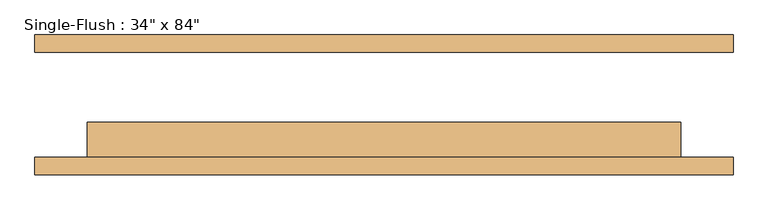
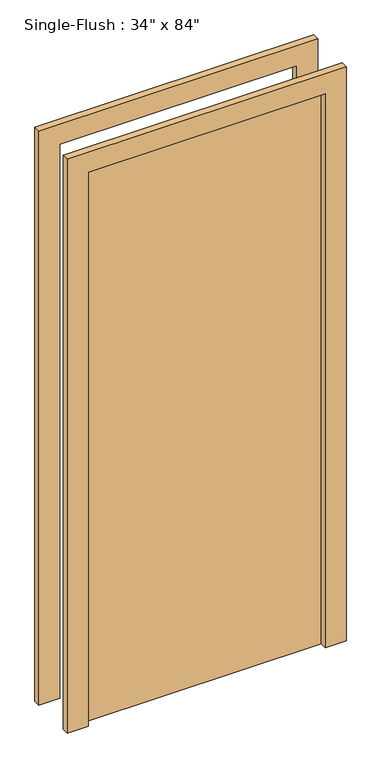
"""IFC4 building model written with IfcOpenShell, lengths in millimetres: door geometry."""

from ifc_helpers import new_model, si_unit, frame, origin, origin_with_axes, place, context, project, spatial, polyline, outline, extrude, source, transform, mapped, element, save


def door_99d96fc5(model_context):
    return source(origin(), model_context, "Body", "SweptSolid", [
        extrude(outline(polyline([(2209.8, -508.0), (0.0, -508.0), (0.0, -431.8), (2133.6, -431.8), (2133.6, 431.8), (0.0, 431.8), (0.0, 508.0), (2209.8, 508.0), (2209.8, -508.0)])), frame((0.0, -101.6, 0.0), z_axis=(0.0, 1.0, 0.0), x_axis=(0.0, 0.0, 1.0)), (0.0, 0.0, 1.0), 25.4),
        extrude(outline(polyline([(2209.8, 508.0), (2209.8, -508.0), (0.0, -508.0), (0.0, -431.8), (2133.6, -431.8), (2133.6, 431.8), (0.0, 431.8), (0.0, 508.0), (2209.8, 508.0)])), frame((0.0, 76.2, 0.0), z_axis=(0.0, 1.0, 0.0), x_axis=(0.0, 0.0, 1.0)), (0.0, 0.0, 1.0), 25.4),
        extrude(outline(polyline([(431.8, -25.4), (431.8, -76.2), (-431.8, -76.2), (-431.8, -25.4), (431.8, -25.4)])), origin_with_axes(), (0.0, 0.0, 1.0), 2133.6),
    ])


if __name__ == "__main__":
    model = new_model("IFC4")
    model_context = context("Model", 3, world=origin())
    ifc_project = project(units=[si_unit("LENGTHUNIT", "METRE", prefix="MILLI")], contexts=[model_context])
    site = spatial("IfcSite", under=ifc_project)
    building = spatial("IfcBuilding", under=site)
    placement = place(None, origin())
    door_shape = door_99d96fc5(model_context)
    element("IfcDoor", 1, ObjectType="Single-Flush : 34\" x 84\"", at=placement, inside=building, context=model_context, shape_type="MappedRepresentation", body=[
        mapped(door_shape, transform((0.0, 0.0, 0.0), x_axis=(1.0, 0.0, 0.0), y_axis=(0.0, 1.0, 0.0), z_axis=(0.0, 0.0, 1.0))),
    ])
    save(model, "model.ifc")

# Revit data of these elements
# Type "Single-Flush : 34\" x 84\""
#   Type Mark = "2"
#   Construction Type Id = "MDOOR"
#   Assembly Code = "C1020"
#   Analytic Construction = "Metal"
#   Thickness = 0' - 2"
#   Heat Transfer Coefficient (U) = 0.651978 BTU/(h·ft²·°F)
#   Height = 7' - 0"
#   Trim Projection Ext = 0' - 1"
#   Trim Projection Int = 0' - 1"
#   Trim Width = 0' - 3"
#   Width = 2' - 10"
#   Define Thermal Properties by = 1
#   Door Material = Door - Panel
#   Frame Material = Door - Frame
#   Visual Light Transmittance = 0
#   Solar Heat Gain Coefficient = 0
#   Function = (empty or 0)
#   Wall Closure = (empty or 0)
# Element 1 (IfcDoor, "Single-Flush : 34\" x 84\"")
#   Materials on its faces: "Door - Frame", "Door - Panel"
# Materials
#   "Door - Panel": class "Wood", colour RGB 210 159 95, transparency 0
#   "Door - Frame": colour RGB 118 70 51, transparency 0
